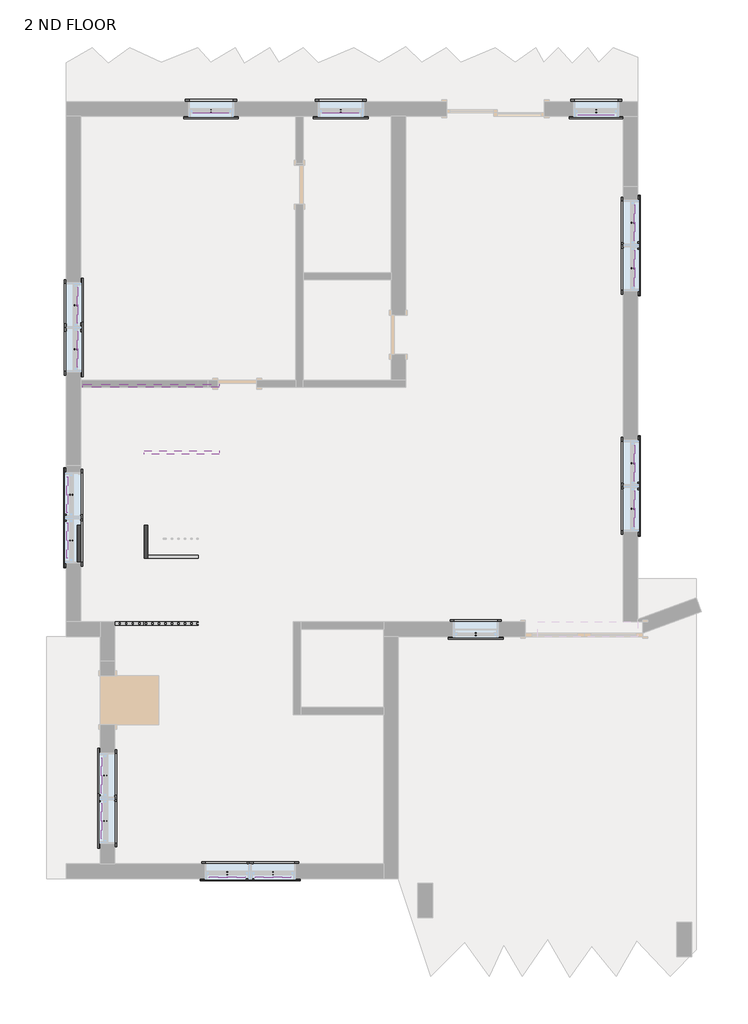
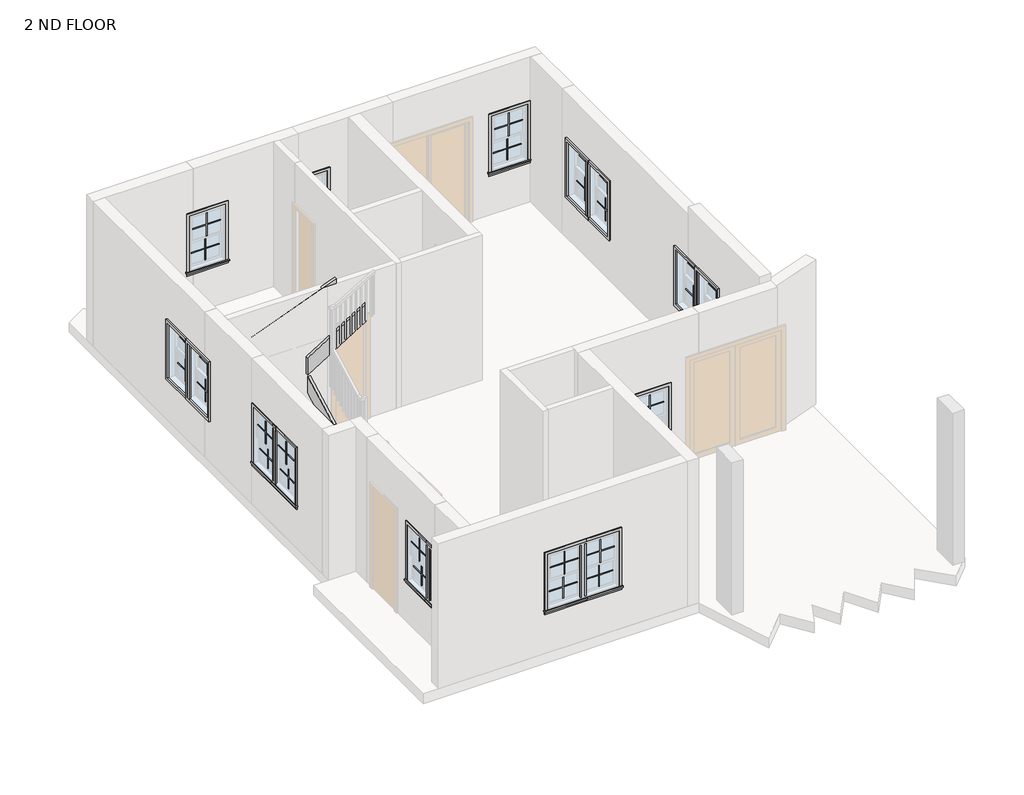
# One storey, part 3 of 3: 64 proxies, 6 members.
"""IFC4 building model written with IfcOpenShell, lengths in millimetres."""

from ifc_helpers import new_model, si_unit, frame, origin, place, context, project, spatial, polyline, outline, extrude, transform, mapped, element, save
from components import muntin_pattern_2x2_muntin_pattern_2x2_5f474966, trim_window_exterior_flat_with_sill_68241f6a, trim_window_interior_flat_picture_frame_d3d93820

model = new_model("IFC4")

# Units and contexts
model_context = context("Model", 3, world=origin())
ifc_project = project(units=[si_unit("LENGTHUNIT", "METRE", prefix="MILLI")], contexts=[model_context])

# Site, building, storey
site = spatial("IfcSite", under=ifc_project)
building = spatial("IfcBuilding", under=site)
storey = spatial("IfcBuildingStorey", under=building, Name="2 ND FLOOR", Elevation=6400.8)

# Proxies
placement = place(None, origin())
muntin_pattern_2x2_muntin_pattern_2x2_shape = muntin_pattern_2x2_muntin_pattern_2x2_5f474966(model_context)
element("IfcBuildingElementProxy", 1, Name="Muntin Pattern_2x2 : Muntin Pattern_2x2", ObjectType="Muntin Pattern_2x2 : Muntin Pattern_2x2", at=placement, inside=storey, context=model_context, shape_type="MappedRepresentation", body=[
    mapped(muntin_pattern_2x2_muntin_pattern_2x2_shape, transform((-20215.5750314, 12584.9473147, 7921.625), x_axis=(-1.0, 0.0, 0.0), y_axis=(0.0, -1.0, 0.0), z_axis=(0.0, 0.0, 1.0))),
])
element("IfcBuildingElementProxy", 2, Name="Muntin Pattern_2x2 : Muntin Pattern_2x2", ObjectType="Muntin Pattern_2x2 : Muntin Pattern_2x2", at=placement, inside=storey, context=model_context, shape_type="MappedRepresentation", body=[
    mapped(muntin_pattern_2x2_muntin_pattern_2x2_shape, transform((-20215.5750314, 12629.3973147, 7391.4), x_axis=(-1.0, 0.0, 0.0), y_axis=(0.0, -1.0, 0.0), z_axis=(0.0, 0.0, 1.0))),
])
element("IfcBuildingElementProxy", 3, Name="Muntin Pattern_2x2 : Muntin Pattern_2x2", ObjectType="Muntin Pattern_2x2 : Muntin Pattern_2x2", at=placement, inside=storey, context=model_context, shape_type="MappedRepresentation", body=[
    mapped(muntin_pattern_2x2_muntin_pattern_2x2_shape, transform((-14208.4750314, 12584.9473147, 7921.625), x_axis=(-1.0, 0.0, 0.0), y_axis=(0.0, -1.0, 0.0), z_axis=(0.0, 0.0, 1.0))),
])
element("IfcBuildingElementProxy", 4, Name="Muntin Pattern_2x2 : Muntin Pattern_2x2", ObjectType="Muntin Pattern_2x2 : Muntin Pattern_2x2", at=placement, inside=storey, context=model_context, shape_type="MappedRepresentation", body=[
    mapped(muntin_pattern_2x2_muntin_pattern_2x2_shape, transform((-14208.4750314, 12629.3973147, 7391.4), x_axis=(-1.0, 0.0, 0.0), y_axis=(0.0, -1.0, 0.0), z_axis=(0.0, 0.0, 1.0))),
])
element("IfcBuildingElementProxy", 5, Name="Muntin Pattern_2x2 : Muntin Pattern_2x2", ObjectType="Muntin Pattern_2x2 : Muntin Pattern_2x2", at=placement, inside=storey, context=model_context, shape_type="MappedRepresentation", body=[
    mapped(muntin_pattern_2x2_muntin_pattern_2x2_shape, transform((-13595.7000314, 10888.3098201, 7921.625), x_axis=(0.0, -1.0, 0.0), y_axis=(1.0, 0.0, 0.0), z_axis=(0.0, 0.0, 1.0))),
])
element("IfcBuildingElementProxy", 6, Name="Muntin Pattern_2x2 : Muntin Pattern_2x2", ObjectType="Muntin Pattern_2x2 : Muntin Pattern_2x2", at=placement, inside=storey, context=model_context, shape_type="MappedRepresentation", body=[
    mapped(muntin_pattern_2x2_muntin_pattern_2x2_shape, transform((-13640.1500314, 10888.3098201, 7391.4), x_axis=(0.0, -1.0, 0.0), y_axis=(1.0, 0.0, 0.0), z_axis=(0.0, 0.0, 1.0))),
])
element("IfcBuildingElementProxy", 7, Name="Muntin Pattern_2x2 : Muntin Pattern_2x2", ObjectType="Muntin Pattern_2x2 : Muntin Pattern_2x2", at=placement, inside=storey, context=model_context, shape_type="MappedRepresentation", body=[
    mapped(muntin_pattern_2x2_muntin_pattern_2x2_shape, transform((-13595.7000314, 10177.1098201, 7921.625), x_axis=(0.0, -1.0, 0.0), y_axis=(1.0, 0.0, 0.0), z_axis=(0.0, 0.0, 1.0))),
])
element("IfcBuildingElementProxy", 8, Name="Muntin Pattern_2x2 : Muntin Pattern_2x2", ObjectType="Muntin Pattern_2x2 : Muntin Pattern_2x2", at=placement, inside=storey, context=model_context, shape_type="MappedRepresentation", body=[
    mapped(muntin_pattern_2x2_muntin_pattern_2x2_shape, transform((-13640.1500314, 10177.1098201, 7391.4), x_axis=(0.0, -1.0, 0.0), y_axis=(1.0, 0.0, 0.0), z_axis=(0.0, 0.0, 1.0))),
])
element("IfcBuildingElementProxy", 9, Name="Muntin Pattern_2x2 : Muntin Pattern_2x2", ObjectType="Muntin Pattern_2x2 : Muntin Pattern_2x2", at=placement, inside=storey, context=model_context, shape_type="MappedRepresentation", body=[
    mapped(muntin_pattern_2x2_muntin_pattern_2x2_shape, transform((-13595.7000314, 7139.8223646, 7921.625), x_axis=(0.0, -1.0, 0.0), y_axis=(1.0, 0.0, 0.0), z_axis=(0.0, 0.0, 1.0))),
])
element("IfcBuildingElementProxy", 10, Name="Muntin Pattern_2x2 : Muntin Pattern_2x2", ObjectType="Muntin Pattern_2x2 : Muntin Pattern_2x2", at=placement, inside=storey, context=model_context, shape_type="MappedRepresentation", body=[
    mapped(muntin_pattern_2x2_muntin_pattern_2x2_shape, transform((-13640.1500314, 7139.8223646, 7391.4), x_axis=(0.0, -1.0, 0.0), y_axis=(1.0, 0.0, 0.0), z_axis=(0.0, 0.0, 1.0))),
])
element("IfcBuildingElementProxy", 11, Name="Muntin Pattern_2x2 : Muntin Pattern_2x2", ObjectType="Muntin Pattern_2x2 : Muntin Pattern_2x2", at=placement, inside=storey, context=model_context, shape_type="MappedRepresentation", body=[
    mapped(muntin_pattern_2x2_muntin_pattern_2x2_shape, transform((-13595.7000314, 6428.6223646, 7921.625), x_axis=(0.0, -1.0, 0.0), y_axis=(1.0, 0.0, 0.0), z_axis=(0.0, 0.0, 1.0))),
])
element("IfcBuildingElementProxy", 12, Name="Muntin Pattern_2x2 : Muntin Pattern_2x2", ObjectType="Muntin Pattern_2x2 : Muntin Pattern_2x2", at=placement, inside=storey, context=model_context, shape_type="MappedRepresentation", body=[
    mapped(muntin_pattern_2x2_muntin_pattern_2x2_shape, transform((-13640.1500314, 6428.6223646, 7391.4), x_axis=(0.0, -1.0, 0.0), y_axis=(1.0, 0.0, 0.0), z_axis=(0.0, 0.0, 1.0))),
])
element("IfcBuildingElementProxy", 13, Name="Muntin Pattern_2x2 : Muntin Pattern_2x2", ObjectType="Muntin Pattern_2x2 : Muntin Pattern_2x2", at=placement, inside=storey, context=model_context, shape_type="MappedRepresentation", body=[
    mapped(muntin_pattern_2x2_muntin_pattern_2x2_shape, transform((-19961.4931686, 697.7473646, 7921.625), x_axis=(-1.0, 0.0, 0.0), y_axis=(0.0, -1.0, 0.0), z_axis=(0.0, 0.0, 1.0))),
])
element("IfcBuildingElementProxy", 14, Name="Muntin Pattern_2x2 : Muntin Pattern_2x2", ObjectType="Muntin Pattern_2x2 : Muntin Pattern_2x2", at=placement, inside=storey, context=model_context, shape_type="MappedRepresentation", body=[
    mapped(muntin_pattern_2x2_muntin_pattern_2x2_shape, transform((-19961.4931686, 742.1973646, 7391.4), x_axis=(-1.0, 0.0, 0.0), y_axis=(0.0, -1.0, 0.0), z_axis=(0.0, 0.0, 1.0))),
])
element("IfcBuildingElementProxy", 15, Name="Muntin Pattern_2x2 : Muntin Pattern_2x2", ObjectType="Muntin Pattern_2x2 : Muntin Pattern_2x2", at=placement, inside=storey, context=model_context, shape_type="MappedRepresentation", body=[
    mapped(muntin_pattern_2x2_muntin_pattern_2x2_shape, transform((-19250.2931686, 697.7473646, 7921.625), x_axis=(-1.0, 0.0, 0.0), y_axis=(0.0, -1.0, 0.0), z_axis=(0.0, 0.0, 1.0))),
])
element("IfcBuildingElementProxy", 16, Name="Muntin Pattern_2x2 : Muntin Pattern_2x2", ObjectType="Muntin Pattern_2x2 : Muntin Pattern_2x2", at=placement, inside=storey, context=model_context, shape_type="MappedRepresentation", body=[
    mapped(muntin_pattern_2x2_muntin_pattern_2x2_shape, transform((-19250.2931686, 742.1973646, 7391.4), x_axis=(-1.0, 0.0, 0.0), y_axis=(0.0, -1.0, 0.0), z_axis=(0.0, 0.0, 1.0))),
])
element("IfcBuildingElementProxy", 17, Name="Muntin Pattern_2x2 : Muntin Pattern_2x2", ObjectType="Muntin Pattern_2x2 : Muntin Pattern_2x2", at=placement, inside=storey, context=model_context, shape_type="MappedRepresentation", body=[
    mapped(muntin_pattern_2x2_muntin_pattern_2x2_shape, transform((-21907.8500314, 2269.3723646, 7921.625), x_axis=(0.0, 1.0, 0.0), y_axis=(-1.0, 0.0, 0.0), z_axis=(0.0, 0.0, 1.0))),
])
element("IfcBuildingElementProxy", 18, Name="Muntin Pattern_2x2 : Muntin Pattern_2x2", ObjectType="Muntin Pattern_2x2 : Muntin Pattern_2x2", at=placement, inside=storey, context=model_context, shape_type="MappedRepresentation", body=[
    mapped(muntin_pattern_2x2_muntin_pattern_2x2_shape, transform((-21863.4000314, 2269.3723646, 7391.4), x_axis=(0.0, 1.0, 0.0), y_axis=(-1.0, 0.0, 0.0), z_axis=(0.0, 0.0, 1.0))),
])
element("IfcBuildingElementProxy", 19, Name="Muntin Pattern_2x2 : Muntin Pattern_2x2", ObjectType="Muntin Pattern_2x2 : Muntin Pattern_2x2", at=placement, inside=storey, context=model_context, shape_type="MappedRepresentation", body=[
    mapped(muntin_pattern_2x2_muntin_pattern_2x2_shape, transform((-21907.8500314, 1558.1723646, 7921.625), x_axis=(0.0, 1.0, 0.0), y_axis=(-1.0, 0.0, 0.0), z_axis=(0.0, 0.0, 1.0))),
])
element("IfcBuildingElementProxy", 20, Name="Muntin Pattern_2x2 : Muntin Pattern_2x2", ObjectType="Muntin Pattern_2x2 : Muntin Pattern_2x2", at=placement, inside=storey, context=model_context, shape_type="MappedRepresentation", body=[
    mapped(muntin_pattern_2x2_muntin_pattern_2x2_shape, transform((-21863.4000314, 1558.1723646, 7391.4), x_axis=(0.0, 1.0, 0.0), y_axis=(-1.0, 0.0, 0.0), z_axis=(0.0, 0.0, 1.0))),
])
element("IfcBuildingElementProxy", 21, Name="Muntin Pattern_2x2 : Muntin Pattern_2x2", ObjectType="Muntin Pattern_2x2 : Muntin Pattern_2x2", at=placement, inside=storey, context=model_context, shape_type="MappedRepresentation", body=[
    mapped(muntin_pattern_2x2_muntin_pattern_2x2_shape, transform((-22441.2502061, 6644.5223643, 7921.625), x_axis=(0.0, 1.0, 0.0), y_axis=(-1.0, 0.0, 0.0), z_axis=(0.0, 0.0, 1.0))),
])
element("IfcBuildingElementProxy", 22, Name="Muntin Pattern_2x2 : Muntin Pattern_2x2", ObjectType="Muntin Pattern_2x2 : Muntin Pattern_2x2", at=placement, inside=storey, context=model_context, shape_type="MappedRepresentation", body=[
    mapped(muntin_pattern_2x2_muntin_pattern_2x2_shape, transform((-22396.8002061, 6644.5223643, 7391.4), x_axis=(0.0, 1.0, 0.0), y_axis=(-1.0, 0.0, 0.0), z_axis=(0.0, 0.0, 1.0))),
])
element("IfcBuildingElementProxy", 23, Name="Muntin Pattern_2x2 : Muntin Pattern_2x2", ObjectType="Muntin Pattern_2x2 : Muntin Pattern_2x2", at=placement, inside=storey, context=model_context, shape_type="MappedRepresentation", body=[
    mapped(muntin_pattern_2x2_muntin_pattern_2x2_shape, transform((-22441.2502061, 5933.3223643, 7921.625), x_axis=(0.0, 1.0, 0.0), y_axis=(-1.0, 0.0, 0.0), z_axis=(0.0, 0.0, 1.0))),
])
element("IfcBuildingElementProxy", 24, Name="Muntin Pattern_2x2 : Muntin Pattern_2x2", ObjectType="Muntin Pattern_2x2 : Muntin Pattern_2x2", at=placement, inside=storey, context=model_context, shape_type="MappedRepresentation", body=[
    mapped(muntin_pattern_2x2_muntin_pattern_2x2_shape, transform((-22396.8002061, 5933.3223643, 7391.4), x_axis=(0.0, 1.0, 0.0), y_axis=(-1.0, 0.0, 0.0), z_axis=(0.0, 0.0, 1.0))),
])
element("IfcBuildingElementProxy", 25, Name="Muntin Pattern_2x2 : Muntin Pattern_2x2", ObjectType="Muntin Pattern_2x2 : Muntin Pattern_2x2", at=placement, inside=storey, context=model_context, shape_type="MappedRepresentation", body=[
    mapped(muntin_pattern_2x2_muntin_pattern_2x2_shape, transform((-22282.5000314, 9599.539033, 7921.625), x_axis=(0.0, -1.0, 0.0), y_axis=(1.0, 0.0, 0.0), z_axis=(0.0, 0.0, 1.0))),
])
element("IfcBuildingElementProxy", 26, Name="Muntin Pattern_2x2 : Muntin Pattern_2x2", ObjectType="Muntin Pattern_2x2 : Muntin Pattern_2x2", at=placement, inside=storey, context=model_context, shape_type="MappedRepresentation", body=[
    mapped(muntin_pattern_2x2_muntin_pattern_2x2_shape, transform((-22326.9500314, 9599.539033, 7391.4), x_axis=(0.0, -1.0, 0.0), y_axis=(1.0, 0.0, 0.0), z_axis=(0.0, 0.0, 1.0))),
])
element("IfcBuildingElementProxy", 27, Name="Muntin Pattern_2x2 : Muntin Pattern_2x2", ObjectType="Muntin Pattern_2x2 : Muntin Pattern_2x2", at=placement, inside=storey, context=model_context, shape_type="MappedRepresentation", body=[
    mapped(muntin_pattern_2x2_muntin_pattern_2x2_shape, transform((-22282.5000314, 8913.739033, 7921.625), x_axis=(0.0, -1.0, 0.0), y_axis=(1.0, 0.0, 0.0), z_axis=(0.0, 0.0, 1.0))),
])
element("IfcBuildingElementProxy", 28, Name="Muntin Pattern_2x2 : Muntin Pattern_2x2", ObjectType="Muntin Pattern_2x2 : Muntin Pattern_2x2", at=placement, inside=storey, context=model_context, shape_type="MappedRepresentation", body=[
    mapped(muntin_pattern_2x2_muntin_pattern_2x2_shape, transform((-22326.9500314, 8913.739033, 7391.4), x_axis=(0.0, -1.0, 0.0), y_axis=(1.0, 0.0, 0.0), z_axis=(0.0, 0.0, 1.0))),
])
element("IfcBuildingElementProxy", 29, Name="Muntin Pattern_2x2 : Muntin Pattern_2x2", ObjectType="Muntin Pattern_2x2 : Muntin Pattern_2x2", at=placement, inside=storey, context=model_context, shape_type="MappedRepresentation", body=[
    mapped(muntin_pattern_2x2_muntin_pattern_2x2_shape, transform((-18193.8494379, 12584.9473147, 7921.625), x_axis=(-1.0, 0.0, 0.0), y_axis=(0.0, -1.0, 0.0), z_axis=(0.0, 0.0, 1.0))),
])
element("IfcBuildingElementProxy", 30, Name="Muntin Pattern_2x2 : Muntin Pattern_2x2", ObjectType="Muntin Pattern_2x2 : Muntin Pattern_2x2", at=placement, inside=storey, context=model_context, shape_type="MappedRepresentation", body=[
    mapped(muntin_pattern_2x2_muntin_pattern_2x2_shape, transform((-18193.8494379, 12629.3973147, 7391.4), x_axis=(-1.0, 0.0, 0.0), y_axis=(0.0, -1.0, 0.0), z_axis=(0.0, 0.0, 1.0))),
])
element("IfcBuildingElementProxy", 31, Name="Muntin Pattern_2x2 : Muntin Pattern_2x2", ObjectType="Muntin Pattern_2x2 : Muntin Pattern_2x2", at=placement, inside=storey, context=model_context, shape_type="MappedRepresentation", body=[
    mapped(muntin_pattern_2x2_muntin_pattern_2x2_shape, transform((-16088.0750314, 4469.6473722, 7568.3384602), x_axis=(-1.0, 0.0, 0.0), y_axis=(0.0, -1.0, 0.0), z_axis=(0.0, 0.0, 1.0))),
])
element("IfcBuildingElementProxy", 32, Name="Muntin Pattern_2x2 : Muntin Pattern_2x2", ObjectType="Muntin Pattern_2x2 : Muntin Pattern_2x2", at=placement, inside=storey, context=model_context, shape_type="MappedRepresentation", body=[
    mapped(muntin_pattern_2x2_muntin_pattern_2x2_shape, transform((-16088.0750314, 4514.0973722, 7038.1134602), x_axis=(-1.0, 0.0, 0.0), y_axis=(0.0, -1.0, 0.0), z_axis=(0.0, 0.0, 1.0))),
])
trim_window_exterior_flat_with_sill_shape = trim_window_exterior_flat_with_sill_68241f6a(model_context)
element("IfcBuildingElementProxy", 33, Name="Trim-Window-Exterior-Flat : with Sill", ObjectType="Trim-Window-Exterior-Flat : with Sill", at=placement, inside=storey, context=model_context, shape_type="MappedRepresentation", body=[
    mapped(trim_window_exterior_flat_with_sill_shape, transform((-20215.5750314, 12550.0223147, 8483.6), x_axis=(1.0, 0.0, 0.0), y_axis=(0.0, 0.0, 1.0), z_axis=(0.0, -1.0, 0.0))),
])
element("IfcBuildingElementProxy", 34, Name="Trim-Window-Exterior-Flat : with Sill", ObjectType="Trim-Window-Exterior-Flat : with Sill", at=placement, inside=storey, context=model_context, shape_type="MappedRepresentation", body=[
    mapped(trim_window_exterior_flat_with_sill_shape, transform((-14208.4750314, 12550.0223147, 8483.6), x_axis=(1.0, 0.0, 0.0), y_axis=(0.0, 0.0, 1.0), z_axis=(0.0, -1.0, 0.0))),
])
element("IfcBuildingElementProxy", 35, Name="Trim-Window-Exterior-Flat : with Sill", ObjectType="Trim-Window-Exterior-Flat : with Sill", at=placement, inside=storey, context=model_context, shape_type="MappedRepresentation", body=[
    mapped(trim_window_exterior_flat_with_sill_shape, transform((-13560.7750314, 10888.3098201, 8483.6), x_axis=(0.0, 1.0, 0.0), y_axis=(0.0, 0.0, 1.0), z_axis=(1.0, 0.0, 0.0))),
])
element("IfcBuildingElementProxy", 36, Name="Trim-Window-Exterior-Flat : with Sill", ObjectType="Trim-Window-Exterior-Flat : with Sill", at=placement, inside=storey, context=model_context, shape_type="MappedRepresentation", body=[
    mapped(trim_window_exterior_flat_with_sill_shape, transform((-13560.7750314, 10177.1098201, 8483.6), x_axis=(0.0, 1.0, 0.0), y_axis=(0.0, 0.0, 1.0), z_axis=(1.0, 0.0, 0.0))),
])
element("IfcBuildingElementProxy", 37, Name="Trim-Window-Exterior-Flat : with Sill", ObjectType="Trim-Window-Exterior-Flat : with Sill", at=placement, inside=storey, context=model_context, shape_type="MappedRepresentation", body=[
    mapped(trim_window_exterior_flat_with_sill_shape, transform((-13560.7750314, 7139.8223646, 8483.6), x_axis=(0.0, 1.0, 0.0), y_axis=(0.0, 0.0, 1.0), z_axis=(1.0, 0.0, 0.0))),
])
element("IfcBuildingElementProxy", 38, Name="Trim-Window-Exterior-Flat : with Sill", ObjectType="Trim-Window-Exterior-Flat : with Sill", at=placement, inside=storey, context=model_context, shape_type="MappedRepresentation", body=[
    mapped(trim_window_exterior_flat_with_sill_shape, transform((-13560.7750314, 6428.6223646, 8483.6), x_axis=(0.0, 1.0, 0.0), y_axis=(0.0, 0.0, 1.0), z_axis=(1.0, 0.0, 0.0))),
])
element("IfcBuildingElementProxy", 39, Name="Trim-Window-Exterior-Flat : with Sill", ObjectType="Trim-Window-Exterior-Flat : with Sill", at=placement, inside=storey, context=model_context, shape_type="MappedRepresentation", body=[
    mapped(trim_window_exterior_flat_with_sill_shape, transform((-19961.4931686, 662.8223646, 8483.6), x_axis=(1.0, 0.0, 0.0), y_axis=(0.0, 0.0, 1.0), z_axis=(0.0, -1.0, 0.0))),
])
element("IfcBuildingElementProxy", 40, Name="Trim-Window-Exterior-Flat : with Sill", ObjectType="Trim-Window-Exterior-Flat : with Sill", at=placement, inside=storey, context=model_context, shape_type="MappedRepresentation", body=[
    mapped(trim_window_exterior_flat_with_sill_shape, transform((-19250.2931686, 662.8223646, 8483.6), x_axis=(1.0, 0.0, 0.0), y_axis=(0.0, 0.0, 1.0), z_axis=(0.0, -1.0, 0.0))),
])
element("IfcBuildingElementProxy", 41, Name="Trim-Window-Exterior-Flat : with Sill", ObjectType="Trim-Window-Exterior-Flat : with Sill", at=placement, inside=storey, context=model_context, shape_type="MappedRepresentation", body=[
    mapped(trim_window_exterior_flat_with_sill_shape, transform((-21942.7750314, 2269.3723646, 8483.6), x_axis=(0.0, -1.0, 0.0), y_axis=(0.0, 0.0, 1.0), z_axis=(-1.0, 0.0, 0.0))),
])
element("IfcBuildingElementProxy", 42, Name="Trim-Window-Exterior-Flat : with Sill", ObjectType="Trim-Window-Exterior-Flat : with Sill", at=placement, inside=storey, context=model_context, shape_type="MappedRepresentation", body=[
    mapped(trim_window_exterior_flat_with_sill_shape, transform((-21942.7750314, 1558.1723646, 8483.6), x_axis=(0.0, -1.0, 0.0), y_axis=(0.0, 0.0, 1.0), z_axis=(-1.0, 0.0, 0.0))),
])
element("IfcBuildingElementProxy", 43, Name="Trim-Window-Exterior-Flat : with Sill", ObjectType="Trim-Window-Exterior-Flat : with Sill", at=placement, inside=storey, context=model_context, shape_type="MappedRepresentation", body=[
    mapped(trim_window_exterior_flat_with_sill_shape, transform((-22476.1752061, 6644.5223643, 8483.6), x_axis=(0.0, -1.0, 0.0), y_axis=(0.0, 0.0, 1.0), z_axis=(-1.0, 0.0, 0.0))),
])
element("IfcBuildingElementProxy", 44, Name="Trim-Window-Exterior-Flat : with Sill", ObjectType="Trim-Window-Exterior-Flat : with Sill", at=placement, inside=storey, context=model_context, shape_type="MappedRepresentation", body=[
    mapped(trim_window_exterior_flat_with_sill_shape, transform((-22476.1752061, 5933.3223643, 8483.6), x_axis=(0.0, -1.0, 0.0), y_axis=(0.0, 0.0, 1.0), z_axis=(-1.0, 0.0, 0.0))),
])
element("IfcBuildingElementProxy", 45, Name="Trim-Window-Exterior-Flat : with Sill", ObjectType="Trim-Window-Exterior-Flat : with Sill", at=placement, inside=storey, context=model_context, shape_type="MappedRepresentation", body=[
    mapped(trim_window_exterior_flat_with_sill_shape, transform((-22247.5750314, 9599.539033, 8483.6), x_axis=(0.0, 1.0, 0.0), y_axis=(0.0, 0.0, 1.0), z_axis=(1.0, 0.0, 0.0))),
])
element("IfcBuildingElementProxy", 46, Name="Trim-Window-Exterior-Flat : with Sill", ObjectType="Trim-Window-Exterior-Flat : with Sill", at=placement, inside=storey, context=model_context, shape_type="MappedRepresentation", body=[
    mapped(trim_window_exterior_flat_with_sill_shape, transform((-22247.5750314, 8913.739033, 8483.6), x_axis=(0.0, 1.0, 0.0), y_axis=(0.0, 0.0, 1.0), z_axis=(1.0, 0.0, 0.0))),
])
element("IfcBuildingElementProxy", 47, Name="Trim-Window-Exterior-Flat : with Sill", ObjectType="Trim-Window-Exterior-Flat : with Sill", at=placement, inside=storey, context=model_context, shape_type="MappedRepresentation", body=[
    mapped(trim_window_exterior_flat_with_sill_shape, transform((-18193.8494379, 12550.0223147, 8483.6), x_axis=(1.0, 0.0, 0.0), y_axis=(0.0, 0.0, 1.0), z_axis=(0.0, -1.0, 0.0))),
])
element("IfcBuildingElementProxy", 48, Name="Trim-Window-Exterior-Flat : with Sill", ObjectType="Trim-Window-Exterior-Flat : with Sill", at=placement, inside=storey, context=model_context, shape_type="MappedRepresentation", body=[
    mapped(trim_window_exterior_flat_with_sill_shape, transform((-16088.0750314, 4434.7223722, 8130.3134602), x_axis=(1.0, 0.0, 0.0), y_axis=(0.0, 0.0, 1.0), z_axis=(0.0, -1.0, 0.0))),
])
trim_window_interior_flat_picture_frame_shape = trim_window_interior_flat_picture_frame_d3d93820(model_context)
element("IfcBuildingElementProxy", 49, Name="Trim-Window-Interior-Flat : Picture Frame", ObjectType="Trim-Window-Interior-Flat : Picture Frame", at=placement, inside=storey, context=model_context, shape_type="MappedRepresentation", body=[
    mapped(trim_window_interior_flat_picture_frame_shape, transform((-20215.5750314, 12778.6223147, 8483.6), x_axis=(-1.0, 0.0, 0.0), y_axis=(0.0, 0.0, 1.0), z_axis=(0.0, 1.0, 0.0))),
])
element("IfcBuildingElementProxy", 50, Name="Trim-Window-Interior-Flat : Picture Frame", ObjectType="Trim-Window-Interior-Flat : Picture Frame", at=placement, inside=storey, context=model_context, shape_type="MappedRepresentation", body=[
    mapped(trim_window_interior_flat_picture_frame_shape, transform((-14208.4750314, 12778.6223147, 8483.6), x_axis=(-1.0, 0.0, 0.0), y_axis=(0.0, 0.0, 1.0), z_axis=(0.0, 1.0, 0.0))),
])
element("IfcBuildingElementProxy", 51, Name="Trim-Window-Interior-Flat : Picture Frame", ObjectType="Trim-Window-Interior-Flat : Picture Frame", at=placement, inside=storey, context=model_context, shape_type="MappedRepresentation", body=[
    mapped(trim_window_interior_flat_picture_frame_shape, transform((-13789.3750314, 10888.3098201, 8483.6), x_axis=(0.0, -1.0, 0.0), y_axis=(0.0, 0.0, 1.0), z_axis=(-1.0, 0.0, 0.0))),
])
element("IfcBuildingElementProxy", 52, Name="Trim-Window-Interior-Flat : Picture Frame", ObjectType="Trim-Window-Interior-Flat : Picture Frame", at=placement, inside=storey, context=model_context, shape_type="MappedRepresentation", body=[
    mapped(trim_window_interior_flat_picture_frame_shape, transform((-13789.3750314, 10177.1098201, 8483.6), x_axis=(0.0, -1.0, 0.0), y_axis=(0.0, 0.0, 1.0), z_axis=(-1.0, 0.0, 0.0))),
])
element("IfcBuildingElementProxy", 53, Name="Trim-Window-Interior-Flat : Picture Frame", ObjectType="Trim-Window-Interior-Flat : Picture Frame", at=placement, inside=storey, context=model_context, shape_type="MappedRepresentation", body=[
    mapped(trim_window_interior_flat_picture_frame_shape, transform((-13789.3750314, 7139.8223646, 8483.6), x_axis=(0.0, -1.0, 0.0), y_axis=(0.0, 0.0, 1.0), z_axis=(-1.0, 0.0, 0.0))),
])
element("IfcBuildingElementProxy", 54, Name="Trim-Window-Interior-Flat : Picture Frame", ObjectType="Trim-Window-Interior-Flat : Picture Frame", at=placement, inside=storey, context=model_context, shape_type="MappedRepresentation", body=[
    mapped(trim_window_interior_flat_picture_frame_shape, transform((-13789.3750314, 6428.6223646, 8483.6), x_axis=(0.0, -1.0, 0.0), y_axis=(0.0, 0.0, 1.0), z_axis=(-1.0, 0.0, 0.0))),
])
element("IfcBuildingElementProxy", 55, Name="Trim-Window-Interior-Flat : Picture Frame", ObjectType="Trim-Window-Interior-Flat : Picture Frame", at=placement, inside=storey, context=model_context, shape_type="MappedRepresentation", body=[
    mapped(trim_window_interior_flat_picture_frame_shape, transform((-19961.4931686, 891.4223646, 8483.6), x_axis=(-1.0, 0.0, 0.0), y_axis=(0.0, 0.0, 1.0), z_axis=(0.0, 1.0, 0.0))),
])
element("IfcBuildingElementProxy", 56, Name="Trim-Window-Interior-Flat : Picture Frame", ObjectType="Trim-Window-Interior-Flat : Picture Frame", at=placement, inside=storey, context=model_context, shape_type="MappedRepresentation", body=[
    mapped(trim_window_interior_flat_picture_frame_shape, transform((-19250.2931686, 891.4223646, 8483.6), x_axis=(-1.0, 0.0, 0.0), y_axis=(0.0, 0.0, 1.0), z_axis=(0.0, 1.0, 0.0))),
])
element("IfcBuildingElementProxy", 57, Name="Trim-Window-Interior-Flat : Picture Frame", ObjectType="Trim-Window-Interior-Flat : Picture Frame", at=placement, inside=storey, context=model_context, shape_type="MappedRepresentation", body=[
    mapped(trim_window_interior_flat_picture_frame_shape, transform((-21714.1750314, 2269.3723646, 8483.6), x_axis=(0.0, 1.0, 0.0), y_axis=(0.0, 0.0, 1.0), z_axis=(1.0, 0.0, 0.0))),
])
element("IfcBuildingElementProxy", 58, Name="Trim-Window-Interior-Flat : Picture Frame", ObjectType="Trim-Window-Interior-Flat : Picture Frame", at=placement, inside=storey, context=model_context, shape_type="MappedRepresentation", body=[
    mapped(trim_window_interior_flat_picture_frame_shape, transform((-21714.1750314, 1558.1723646, 8483.6), x_axis=(0.0, 1.0, 0.0), y_axis=(0.0, 0.0, 1.0), z_axis=(1.0, 0.0, 0.0))),
])
element("IfcBuildingElementProxy", 59, Name="Trim-Window-Interior-Flat : Picture Frame", ObjectType="Trim-Window-Interior-Flat : Picture Frame", at=placement, inside=storey, context=model_context, shape_type="MappedRepresentation", body=[
    mapped(trim_window_interior_flat_picture_frame_shape, transform((-22247.5752061, 6644.5223643, 8483.6), x_axis=(0.0, 1.0, 0.0), y_axis=(0.0, 0.0, 1.0), z_axis=(1.0, 0.0, 0.0))),
])
element("IfcBuildingElementProxy", 60, Name="Trim-Window-Interior-Flat : Picture Frame", ObjectType="Trim-Window-Interior-Flat : Picture Frame", at=placement, inside=storey, context=model_context, shape_type="MappedRepresentation", body=[
    mapped(trim_window_interior_flat_picture_frame_shape, transform((-22247.5752061, 5933.3223643, 8483.6), x_axis=(0.0, 1.0, 0.0), y_axis=(0.0, 0.0, 1.0), z_axis=(1.0, 0.0, 0.0))),
])
element("IfcBuildingElementProxy", 61, Name="Trim-Window-Interior-Flat : Picture Frame", ObjectType="Trim-Window-Interior-Flat : Picture Frame", at=placement, inside=storey, context=model_context, shape_type="MappedRepresentation", body=[
    mapped(trim_window_interior_flat_picture_frame_shape, transform((-22476.1750314, 9599.539033, 8483.6), x_axis=(0.0, -1.0, 0.0), y_axis=(0.0, 0.0, 1.0), z_axis=(-1.0, 0.0, 0.0))),
])
element("IfcBuildingElementProxy", 62, Name="Trim-Window-Interior-Flat : Picture Frame", ObjectType="Trim-Window-Interior-Flat : Picture Frame", at=placement, inside=storey, context=model_context, shape_type="MappedRepresentation", body=[
    mapped(trim_window_interior_flat_picture_frame_shape, transform((-22476.1750314, 8913.739033, 8483.6), x_axis=(0.0, -1.0, 0.0), y_axis=(0.0, 0.0, 1.0), z_axis=(-1.0, 0.0, 0.0))),
])
element("IfcBuildingElementProxy", 63, Name="Trim-Window-Interior-Flat : Picture Frame", ObjectType="Trim-Window-Interior-Flat : Picture Frame", at=placement, inside=storey, context=model_context, shape_type="MappedRepresentation", body=[
    mapped(trim_window_interior_flat_picture_frame_shape, transform((-18193.8494379, 12778.6223147, 8483.6), x_axis=(-1.0, 0.0, 0.0), y_axis=(0.0, 0.0, 1.0), z_axis=(0.0, 1.0, 0.0))),
])
element("IfcBuildingElementProxy", 64, Name="Trim-Window-Interior-Flat : Picture Frame", ObjectType="Trim-Window-Interior-Flat : Picture Frame", at=placement, inside=storey, context=model_context, shape_type="MappedRepresentation", body=[
    mapped(trim_window_interior_flat_picture_frame_shape, transform((-16088.0750314, 4663.3223722, 8130.3134602), x_axis=(-1.0, 0.0, 0.0), y_axis=(0.0, 0.0, 1.0), z_axis=(0.0, 1.0, 0.0))),
])

# Members
element("IfcMember", 65, ObjectType="Stringer - 2\" Width", at=placement, inside=storey, context=model_context, shape_type="SweptSolid", body=[
    extrude(outline(polyline([(6531.3252239, -20418.7750314), (6853.6815263, -20418.7750314), (7147.7746925, -21273.045657), (7147.7746925, -22209.4139641), (6531.3252239, -20418.7750314)])), frame((0.0, 4612.5223646, 0.0), z_axis=(0.0, 1.0, 0.0), x_axis=(0.0, 0.0, 1.0)), (0.0, 0.0, 1.0), 50.8),
])
element("IfcMember", 66, ObjectType="Stringer - 2\" Width", at=placement, inside=storey, context=model_context, shape_type="SweptSolid", body=[
    extrude(outline(polyline([(4688.0958922, 7160.9121693), (7646.6888829, 8729.8629977), (8297.2722107, 8729.8629977), (5338.67922, 7160.9121693), (4688.0958922, 7160.9121693)])), frame((-22298.3752061, 0.0, 0.0), z_axis=(1.0, 0.0, 0.0), x_axis=(0.0, 1.0, 0.0)), (0.0, 0.0, 1.0), 50.8),
])
element("IfcMember", 67, ObjectType="Stringer - 2\" Width", at=placement, inside=storey, context=model_context, shape_type="SweptSolid", body=[
    extrude(outline(polyline([(8742.404746, -21363.7701417), (9231.5206787, -20088.5750314), (9557.9726538, -20088.5750314), (8742.404746, -22214.8770766), (8742.404746, -21363.7701417)])), frame((0.0, 8320.9223646, 0.0), z_axis=(0.0, 1.0, 0.0), x_axis=(0.0, 0.0, 1.0)), (0.0, 0.0, 1.0), 50.8),
])
element("IfcMember", 68, ObjectType="Stringer - 2\" Width", at=placement, inside=storey, context=model_context, shape_type="SweptSolid", body=[
    extrude(outline(polyline([(6432.3282995, -20418.7750314), (6793.6106437, -20418.7750314), (7294.683371, -21206.1750314), (6933.4010268, -21206.1750314), (6432.3282995, -20418.7750314)])), frame((0.0, 5653.9223646, 0.0), z_axis=(0.0, 1.0, 0.0), x_axis=(0.0, 0.0, 1.0)), (0.0, 0.0, 1.0), 50.8),
])
element("IfcMember", 69, ObjectType="Stringer - 2\" Width", at=placement, inside=storey, context=model_context, shape_type="SweptSolid", body=[
    extrude(outline(polyline([(5653.9223646, 7328.0865642), (5653.9223646, 7673.0928743), (7279.5223646, 8535.1534804), (7279.5223646, 8190.1471702), (5653.9223646, 7328.0865642)])), frame((-21256.9750314, 0.0, 0.0), z_axis=(1.0, 0.0, 0.0), x_axis=(0.0, 1.0, 0.0)), (0.0, 0.0, 1.0), 50.8),
])
element("IfcMember", 70, ObjectType="Stringer - 2\" Width", at=placement, inside=storey, context=model_context, shape_type="SweptSolid", body=[
    extrude(outline(polyline([(8925.4057942, -21256.9750314), (8567.1538932, -21256.9750314), (9288.8127167, -20088.5750314), (9647.0646178, -20088.5750314), (8925.4057942, -21256.9750314)])), frame((0.0, 7279.5223646, 0.0), z_axis=(0.0, 1.0, 0.0), x_axis=(0.0, 0.0, 1.0)), (0.0, 0.0, 1.0), 50.8),
])

save(model, "model.ifc")

# Revit data of these elements
# Type "Muntin Pattern_2x2 : Muntin Pattern_2x2"
#   Width [instance default] = 4' - 0"
#   Thickness = 0' - 0 1/2"
#   Height [instance default] = 4' - 0"
#   Distance = 0' - 0 3/4"
#   Interior Material [instance default] = none
#   Exterior Material [instance default] = none
#   Default Elevation = 0
# Type "Trim-Window-Exterior-Flat : with Sill"
#   Trim Width = 0' - 2 1/4"
#   Trim Thickness_Picture Frame = 0' - 1 1/4"
#   Trim Thickness_with Sill = 0' - 0 3/4"
#   Sill Thickness = 0' - 1 1/4"
#   Opening Width [instance default] = 2' - 0"
#   Opening Height [instance default] = 3' - 0"
#   Default Elevation = 4' - 0"
#   Sill = yes
#   Picture Frame = no
#   Trim Material [instance default] = none
# Type "Trim-Window-Interior-Flat : Picture Frame"
#   Trim Thickness_Picture Frame = 0' - 1 1/4"
#   Trim Width = 0' - 2 1/4"
#   Trim Thickness_with Sill = 0' - 0 3/4"
#   Sill Thickness = 0' - 1 1/4"
#   Opening Width [instance default] = 2' - 0"
#   Opening Height [instance default] = 3' - 0"
#   Default Elevation = 4' - 0"
#   Sill = no
#   Picture Frame = yes
#   Trim Material [instance default] = none
# Elements 1, 2, 3, 4, 5, 6, 7, 8, 9, 10, 11, 12, 13, 14, 15, 16, 17, 18, 19, 20, 21, 22, 23, 24, 25, 26, 27, 28, 29, 30, 31, 32 (IfcBuildingElementProxy, "Muntin Pattern_2x2 : Muntin Pattern_2x2")
#   Width = 1' - 10"
#   Height = 1' - 7 1/8"
#   Interior Material = Wood - Stained
#   Exterior Material = Clad - White
#   Phase Created = New Construction
#   Materials on its faces: "Clad - White", "Wood - Stained"
# Elements 33, 34, 35, 36, 37, 38, 39, 40, 41, 42, 43, 44, 45, 46, 47, 48 (IfcBuildingElementProxy, "Trim-Window-Exterior-Flat : with Sill")
#   Opening Width = 2' - 4"
#   Opening Height = 3' - 10"
#   Trim Material = Clad - White
#   Phase Created = New Construction
#   Materials on its faces: "Clad - White"
# Elements 49, 50, 51, 52, 53, 54, 55, 56, 57, 58, 59, 60, 61, 62, 63, 64 (IfcBuildingElementProxy, "Trim-Window-Interior-Flat : Picture Frame")
#   Opening Width = 2' - 4"
#   Opening Height = 3' - 10"
#   Trim Material = Wood - Stained
#   Phase Created = New Construction
#   Materials on its faces: "Wood - Stained"
# Elements 65, 66, 67, 68, 69, 70 (IfcMember, "Stringer - 2\" Width")
#   Phase Created = New Construction
# Materials
#   "Clad - White": class "Wood", colour RGB 242 242 238, transparency 0, Cost = 0
#   "Wood - Stained": class "Wood", colour RGB 224 178 126, transparency 0, Cost = 0
